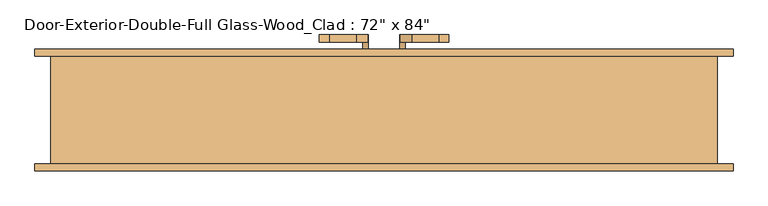
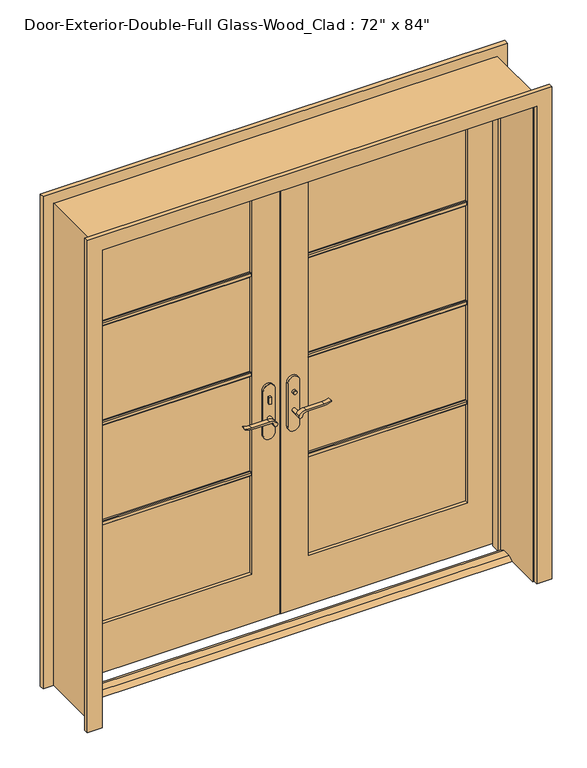
"""IFC4 building model written with IfcOpenShell, lengths in millimetres: door geometry."""

from ifc_helpers import new_model, si_unit, point, frame, frame_2d, origin, place, context, project, spatial, polyline, circle_curve, trimmed, segment, composite_curve, outline, extrude, faceted_brep, source, transform, mapped, element, save


def door_c1904fbe(model_context):
    return source(origin(), model_context, "Body", "SolidModel", [
        extrude(outline(polyline([(19.05, 12.7), (53.975, 12.7), (79.375, 0.0), (-6.35, 0.0), (19.05, 12.7)])), frame((-914.4, 0.0, 0.0), z_axis=(1.0, 0.0, 0.0), x_axis=(0.0, 1.0, 0.0)), (0.0, 0.0, 1.0), 1828.8),
        extrude(outline(polyline([(-47.4019111, 94.3), (-57.4019111, 94.3), (-57.4019111, 104.3), (-47.4019111, 104.3), (-47.4019111, 94.3)])), frame((0.0, 0.0, 981.9), z_axis=(0.0, 0.0, 1.0), x_axis=(1.0, 0.0, 0.0)), (0.0, 0.0, 1.0), 30.0),
        extrude(outline(composite_curve([segment(trimmed(circle_curve(frame_2d((996.9, -52.4019111)), 8.0), [point((996.9, -60.4019111))], [point((996.9, -44.4019111))], False, "CARTESIAN"), True, "CONTINUOUS"), segment(trimmed(circle_curve(frame_2d((996.9, -52.4019111)), 8.0), [point((996.9, -44.4019111))], [point((996.9, -60.4019111))], False, "CARTESIAN"), True, "CONTINUOUS")], self_intersect=False)), frame((0.0, 159.225, 0.0), z_axis=(0.0, 1.0, 0.0), x_axis=(0.0, 0.0, 1.0)), (0.0, 0.0, 1.0), 10.0),
        extrude(outline(composite_curve([segment(trimmed(circle_curve(frame_2d((897.1555521, -76.0694241)), 37.2832219), [point((919.0523287, -45.8937749))], [point((934.4, -77.7693445))], False, "CARTESIAN"), True, "CONTINUOUS"), segment(polyline([(934.4, -77.7693445), (934.4, -154.045502)]), True, "CONTINUOUS"), segment(trimmed(circle_curve(frame_2d((1017.6850638, -153.9791202)), 83.2850902), [point((934.4, -154.045502))], [point((939.4, -182.4019111))], True, "CARTESIAN"), True, "CONTINUOUS"), segment(polyline([(939.4, -182.4019111), (936.6135558, -182.4019111)]), True, "CONTINUOUS"), segment(trimmed(circle_curve(frame_2d((986.6709207, -150.4622499)), 59.3791355), [point((936.6135558, -182.4019111))], [point((927.4, -154.045502))], False, "CARTESIAN"), True, "CONTINUOUS"), segment(polyline([(927.4, -154.045502), (927.4, -77.7881013)]), True, "CONTINUOUS"), segment(trimmed(circle_curve(frame_2d((909.2738613, -77.7881013)), 18.1261387), [point((927.4, -77.7881013))], [point((914.4, -60.4019111))], True, "CARTESIAN"), True, "CONTINUOUS"), segment(trimmed(circle_curve(frame_2d((914.4, -52.4019111)), 8.0), [point((914.4, -60.4019111))], [point((919.0523287, -45.8937749))], False, "CARTESIAN"), True, "CONTINUOUS")], self_intersect=False)), frame((0.0, 54.3, 0.0), z_axis=(0.0, 1.0, 0.0), x_axis=(0.0, 0.0, 1.0)), (0.0, 0.0, 1.0), 20.0),
        extrude(outline(composite_curve([segment(trimmed(circle_curve(frame_2d((914.4, -52.4019111)), 8.0), [point((914.3999903, -60.4019111))], [point((919.0523287, -45.8937749))], False, "CARTESIAN"), True, "CONTINUOUS"), segment(trimmed(circle_curve(frame_2d((897.1555521, -76.0694241)), 37.2832219), [point((919.0523287, -45.8937749))], [point((934.4, -77.7693445))], False, "CARTESIAN"), True, "CONTINUOUS"), segment(polyline([(934.4, -77.7693445), (934.4, -154.045502)]), True, "CONTINUOUS"), segment(trimmed(circle_curve(frame_2d((1017.6850638, -153.9791202)), 83.2850902), [point((934.4, -154.045502))], [point((939.4, -182.4019111))], True, "CARTESIAN"), True, "CONTINUOUS"), segment(polyline([(939.4, -182.4019111), (936.6135558, -182.4019111)]), True, "CONTINUOUS"), segment(trimmed(circle_curve(frame_2d((986.6709207, -150.4622499)), 59.3791355), [point((936.6135558, -182.4019111))], [point((927.4, -154.045502))], False, "CARTESIAN"), True, "CONTINUOUS"), segment(polyline([(927.4, -154.045502), (927.4, -77.788099)]), True, "CONTINUOUS"), segment(trimmed(circle_curve(frame_2d((909.2738682, -77.788099)), 18.1261318), [point((927.4, -77.788099))], [point((914.3999903, -60.4019111))], True, "CARTESIAN"), True, "CONTINUOUS")], self_intersect=False)), frame((0.0, 189.225, 0.0), z_axis=(0.0, 1.0, 0.0), x_axis=(0.0, 0.0, 1.0)), (0.0, 0.0, 1.0), 20.0),
        extrude(outline(composite_curve([segment(trimmed(circle_curve(frame_2d((914.4, -52.4019111)), 8.0), [point((914.4, -60.4019111))], [point((914.4, -44.4019111))], False, "CARTESIAN"), True, "CONTINUOUS"), segment(trimmed(circle_curve(frame_2d((914.4, -52.4019111)), 8.0), [point((914.4, -44.4019111))], [point((914.4, -60.4019111))], False, "CARTESIAN"), True, "CONTINUOUS")], self_intersect=False)), frame((0.0, 74.3, 0.0), z_axis=(0.0, 1.0, 0.0), x_axis=(0.0, 0.0, 1.0)), (0.0, 0.0, 1.0), 30.0),
        extrude(outline(composite_curve([segment(trimmed(circle_curve(frame_2d((914.4, -52.4019111)), 8.0), [point((914.4, -60.4019111))], [point((914.4, -44.4019111))], False, "CARTESIAN"), True, "CONTINUOUS"), segment(trimmed(circle_curve(frame_2d((914.4, -52.4019111)), 8.0), [point((914.4, -44.4019111))], [point((914.4, -60.4019111))], False, "CARTESIAN"), True, "CONTINUOUS")], self_intersect=False)), frame((0.0, 159.225, 0.0), z_axis=(0.0, 1.0, 0.0), x_axis=(0.0, 0.0, 1.0)), (0.0, 0.0, 1.0), 30.0),
        extrude(outline(composite_curve([segment(polyline([(844.4, -27.4019111), (1039.4, -27.4019111)]), True, "CONTINUOUS"), segment(trimmed(circle_curve(frame_2d((1039.4, -52.4019111)), 25.0), [point((1039.4, -27.4019111))], [point((1039.4, -77.4019111))], False, "CARTESIAN"), True, "CONTINUOUS"), segment(polyline([(1039.4, -77.4019111), (844.4, -77.4019111)]), True, "CONTINUOUS"), segment(trimmed(circle_curve(frame_2d((844.4, -52.4019111)), 25.0), [point((844.4, -77.4019111))], [point((844.4, -27.4019111))], False, "CARTESIAN"), True, "CONTINUOUS")], self_intersect=False)), frame((0.0, 104.3, 0.0), z_axis=(0.0, 1.0, 0.0), x_axis=(0.0, 0.0, 1.0)), (0.0, 0.0, 1.0), 10.0),
        extrude(outline(composite_curve([segment(polyline([(844.4, -27.4019111), (1039.4, -27.4019111)]), True, "CONTINUOUS"), segment(trimmed(circle_curve(frame_2d((1039.4, -52.4019111)), 25.0), [point((1039.4, -27.4019111))], [point((1039.4, -77.4019111))], False, "CARTESIAN"), True, "CONTINUOUS"), segment(polyline([(1039.4, -77.4019111), (844.4, -77.4019111)]), True, "CONTINUOUS"), segment(trimmed(circle_curve(frame_2d((844.4, -52.4019111)), 25.0), [point((844.4, -77.4019111))], [point((844.4, -27.4019111))], False, "CARTESIAN"), True, "CONTINUOUS")], self_intersect=False)), frame((0.0, 149.225, 0.0), z_axis=(0.0, 1.0, 0.0), x_axis=(0.0, 0.0, 1.0)), (0.0, 0.0, 1.0), 10.0),
        extrude(outline(polyline([(47.3875, 169.225), (57.3875, 169.225), (57.3875, 159.225), (47.3875, 159.225), (47.3875, 169.225)])), frame((0.0, 0.0, 981.9), z_axis=(0.0, 0.0, 1.0), x_axis=(1.0, 0.0, 0.0)), (0.0, 0.0, 1.0), 30.0),
        extrude(outline(composite_curve([segment(trimmed(circle_curve(frame_2d((996.9, 52.3875)), 8.0), [point((996.9, 60.3875))], [point((996.9, 44.3875))], False, "CARTESIAN"), True, "CONTINUOUS"), segment(trimmed(circle_curve(frame_2d((996.9, 52.3875)), 8.0), [point((996.9, 44.3875))], [point((996.9, 60.3875))], False, "CARTESIAN"), True, "CONTINUOUS")], self_intersect=False)), frame((0.0, 94.3, 0.0), z_axis=(0.0, 1.0, 0.0), x_axis=(0.0, 0.0, 1.0)), (0.0, 0.0, 1.0), 10.0),
        extrude(outline(composite_curve([segment(trimmed(circle_curve(frame_2d((914.4, 52.3875)), 8.0), [point((919.0523287, 45.8793637))], [point((914.4, 60.3875))], False, "CARTESIAN"), True, "CONTINUOUS"), segment(trimmed(circle_curve(frame_2d((909.2738613, 77.7736901)), 18.1261387), [point((914.4, 60.3875))], [point((927.4, 77.7736901))], True, "CARTESIAN"), True, "CONTINUOUS"), segment(polyline([(927.4, 77.7736901), (927.4, 154.0310909)]), True, "CONTINUOUS"), segment(trimmed(circle_curve(frame_2d((986.6709207, 150.4478388)), 59.3791355), [point((927.4, 154.0310909))], [point((936.6135558, 182.3875))], False, "CARTESIAN"), True, "CONTINUOUS"), segment(polyline([(936.6135558, 182.3875), (939.4, 182.3875)]), True, "CONTINUOUS"), segment(trimmed(circle_curve(frame_2d((1017.6850638, 153.9647091)), 83.2850902), [point((939.4, 182.3875))], [point((934.4, 154.0310909))], True, "CARTESIAN"), True, "CONTINUOUS"), segment(polyline([(934.4, 154.0310909), (934.4, 77.7549333)]), True, "CONTINUOUS"), segment(trimmed(circle_curve(frame_2d((897.1555521, 76.0550129)), 37.2832219), [point((934.4, 77.7549333))], [point((919.0523287, 45.8793637))], False, "CARTESIAN"), True, "CONTINUOUS")], self_intersect=False)), frame((0.0, 189.225, 0.0), z_axis=(0.0, 1.0, 0.0), x_axis=(0.0, 0.0, 1.0)), (0.0, 0.0, 1.0), 20.0),
        extrude(outline(composite_curve([segment(trimmed(circle_curve(frame_2d((909.2738682, 77.7736878)), 18.1261318), [point((914.3999903, 60.3875))], [point((927.4, 77.7736878))], True, "CARTESIAN"), True, "CONTINUOUS"), segment(polyline([(927.4, 77.7736878), (927.4, 154.0310909)]), True, "CONTINUOUS"), segment(trimmed(circle_curve(frame_2d((986.6709207, 150.4478388)), 59.3791355), [point((927.4, 154.0310909))], [point((936.6135558, 182.3875))], False, "CARTESIAN"), True, "CONTINUOUS"), segment(polyline([(936.6135558, 182.3875), (939.4, 182.3875)]), True, "CONTINUOUS"), segment(trimmed(circle_curve(frame_2d((1017.6850638, 153.9647091)), 83.2850902), [point((939.4, 182.3875))], [point((934.4, 154.0310909))], True, "CARTESIAN"), True, "CONTINUOUS"), segment(polyline([(934.4, 154.0310909), (934.4, 77.7549333)]), True, "CONTINUOUS"), segment(trimmed(circle_curve(frame_2d((897.1555521, 76.0550129)), 37.2832219), [point((934.4, 77.7549333))], [point((919.0523287, 45.8793637))], False, "CARTESIAN"), True, "CONTINUOUS"), segment(trimmed(circle_curve(frame_2d((914.4, 52.3875)), 8.0), [point((919.0523287, 45.8793637))], [point((914.3999903, 60.3875))], False, "CARTESIAN"), True, "CONTINUOUS")], self_intersect=False)), frame((0.0, 54.3, 0.0), z_axis=(0.0, 1.0, 0.0), x_axis=(0.0, 0.0, 1.0)), (0.0, 0.0, 1.0), 20.0),
        extrude(outline(composite_curve([segment(trimmed(circle_curve(frame_2d((914.4, 52.3875)), 8.0), [point((914.4, 60.3875))], [point((914.4, 44.3875))], False, "CARTESIAN"), True, "CONTINUOUS"), segment(trimmed(circle_curve(frame_2d((914.4, 52.3875)), 8.0), [point((914.4, 44.3875))], [point((914.4, 60.3875))], False, "CARTESIAN"), True, "CONTINUOUS")], self_intersect=False)), frame((0.0, 159.225, 0.0), z_axis=(0.0, 1.0, 0.0), x_axis=(0.0, 0.0, 1.0)), (0.0, 0.0, 1.0), 30.0),
        extrude(outline(composite_curve([segment(trimmed(circle_curve(frame_2d((914.4, 52.3875)), 8.0), [point((914.4, 60.3875))], [point((914.4, 44.3875))], False, "CARTESIAN"), True, "CONTINUOUS"), segment(trimmed(circle_curve(frame_2d((914.4, 52.3875)), 8.0), [point((914.4, 44.3875))], [point((914.4, 60.3875))], False, "CARTESIAN"), True, "CONTINUOUS")], self_intersect=False)), frame((0.0, 74.3, 0.0), z_axis=(0.0, 1.0, 0.0), x_axis=(0.0, 0.0, 1.0)), (0.0, 0.0, 1.0), 30.0),
        extrude(outline(composite_curve([segment(trimmed(circle_curve(frame_2d((844.4, 52.3875)), 25.0), [point((844.4, 27.3875))], [point((844.4, 77.3875))], False, "CARTESIAN"), True, "CONTINUOUS"), segment(polyline([(844.4, 77.3875), (1039.4, 77.3875)]), True, "CONTINUOUS"), segment(trimmed(circle_curve(frame_2d((1039.4, 52.3875)), 25.0), [point((1039.4, 77.3875))], [point((1039.4, 27.3875))], False, "CARTESIAN"), True, "CONTINUOUS"), segment(polyline([(1039.4, 27.3875), (844.4, 27.3875)]), True, "CONTINUOUS")], self_intersect=False)), frame((0.0, 149.225, 0.0), z_axis=(0.0, 1.0, 0.0), x_axis=(0.0, 0.0, 1.0)), (0.0, 0.0, 1.0), 10.0),
        extrude(outline(composite_curve([segment(trimmed(circle_curve(frame_2d((844.4, 52.3875)), 25.0), [point((844.4, 27.3875))], [point((844.4, 77.3875))], False, "CARTESIAN"), True, "CONTINUOUS"), segment(polyline([(844.4, 77.3875), (1039.4, 77.3875)]), True, "CONTINUOUS"), segment(trimmed(circle_curve(frame_2d((1039.4, 52.3875)), 25.0), [point((1039.4, 77.3875))], [point((1039.4, 27.3875))], False, "CARTESIAN"), True, "CONTINUOUS"), segment(polyline([(1039.4, 27.3875), (844.4, 27.3875)]), True, "CONTINUOUS")], self_intersect=False)), frame((0.0, 104.3, 0.0), z_axis=(0.0, 1.0, 0.0), x_axis=(0.0, 0.0, 1.0)), (0.0, 0.0, 1.0), 10.0),
        extrude(outline(polyline([(128.27, 1578.371875), (128.27, 1559.321875), (121.92, 1559.321875), (118.745, 1562.496875), (118.745, 1575.196875), (121.92, 1578.371875), (128.27, 1578.371875)])), frame((120.65, 0.0, 0.0), z_axis=(1.0, 0.0, 0.0), x_axis=(0.0, 1.0, 0.0)), (0.0, 0.0, 1.0), 673.1),
        extrude(outline(polyline([(128.27, 1132.68125), (128.27, 1113.63125), (121.92, 1113.63125), (118.745, 1116.80625), (118.745, 1129.50625), (121.92, 1132.68125), (128.27, 1132.68125)])), frame((120.65, 0.0, 0.0), z_axis=(1.0, 0.0, 0.0), x_axis=(0.0, 1.0, 0.0)), (0.0, 0.0, 1.0), 673.1),
        extrude(outline(polyline([(128.27, 686.990625), (128.27, 667.940625), (121.92, 667.940625), (118.745, 671.115625), (118.745, 683.815625), (121.92, 686.990625), (128.27, 686.990625)])), frame((120.65, 0.0, 0.0), z_axis=(1.0, 0.0, 0.0), x_axis=(0.0, 1.0, 0.0)), (0.0, 0.0, 1.0), 673.1),
        extrude(outline(polyline([(135.255, 1578.371875), (141.605, 1578.371875), (144.78, 1575.196875), (144.78, 1562.496875), (141.605, 1559.321875), (135.255, 1559.321875), (135.255, 1578.371875)])), frame((-793.75, 0.0, 0.0), z_axis=(1.0, 0.0, 0.0), x_axis=(0.0, 1.0, 0.0)), (0.0, 0.0, 1.0), 673.1),
        extrude(outline(polyline([(135.255, 1132.68125), (141.605, 1132.68125), (144.78, 1129.50625), (144.78, 1116.80625), (141.605, 1113.63125), (135.255, 1113.63125), (135.255, 1132.68125)])), frame((-793.75, 0.0, 0.0), z_axis=(1.0, 0.0, 0.0), x_axis=(0.0, 1.0, 0.0)), (0.0, 0.0, 1.0), 673.1),
        extrude(outline(polyline([(135.255, 686.990625), (141.605, 686.990625), (144.78, 683.815625), (144.78, 671.115625), (141.605, 667.940625), (135.255, 667.940625), (135.255, 686.990625)])), frame((-793.75, 0.0, 0.0), z_axis=(1.0, 0.0, 0.0), x_axis=(0.0, 1.0, 0.0)), (0.0, 0.0, 1.0), 673.1),
        extrude(outline(polyline([(135.255, 1578.371875), (141.605, 1578.371875), (144.78, 1575.196875), (144.78, 1562.496875), (141.605, 1559.321875), (135.255, 1559.321875), (135.255, 1578.371875)])), frame((120.65, 0.0, 0.0), z_axis=(1.0, 0.0, 0.0), x_axis=(0.0, 1.0, 0.0)), (0.0, 0.0, 1.0), 673.1),
        extrude(outline(polyline([(135.255, 1132.68125), (141.605, 1132.68125), (144.78, 1129.50625), (144.78, 1116.80625), (141.605, 1113.63125), (135.255, 1113.63125), (135.255, 1132.68125)])), frame((120.65, 0.0, 0.0), z_axis=(1.0, 0.0, 0.0), x_axis=(0.0, 1.0, 0.0)), (0.0, 0.0, 1.0), 673.1),
        extrude(outline(polyline([(135.255, 686.990625), (141.605, 686.990625), (144.78, 683.815625), (144.78, 671.115625), (141.605, 667.940625), (135.255, 667.940625), (135.255, 686.990625)])), frame((120.65, 0.0, 0.0), z_axis=(1.0, 0.0, 0.0), x_axis=(0.0, 1.0, 0.0)), (0.0, 0.0, 1.0), 673.1),
        extrude(outline(polyline([(128.27, 1578.371875), (128.27, 1559.321875), (121.92, 1559.321875), (118.745, 1562.496875), (118.745, 1575.196875), (121.92, 1578.371875), (128.27, 1578.371875)])), frame((-793.75, 0.0, 0.0), z_axis=(1.0, 0.0, 0.0), x_axis=(0.0, 1.0, 0.0)), (0.0, 0.0, 1.0), 673.1),
        extrude(outline(polyline([(128.27, 1132.68125), (128.27, 1113.63125), (121.92, 1113.63125), (118.745, 1116.80625), (118.745, 1129.50625), (121.92, 1132.68125), (128.27, 1132.68125)])), frame((-793.75, 0.0, 0.0), z_axis=(1.0, 0.0, 0.0), x_axis=(0.0, 1.0, 0.0)), (0.0, 0.0, 1.0), 673.1),
        extrude(outline(polyline([(128.27, 686.990625), (128.27, 667.940625), (121.92, 667.940625), (118.745, 671.115625), (118.745, 683.815625), (121.92, 686.990625), (128.27, 686.990625)])), frame((-793.75, 0.0, 0.0), z_axis=(1.0, 0.0, 0.0), x_axis=(0.0, 1.0, 0.0)), (0.0, 0.0, 1.0), 673.1),
        extrude(outline(polyline([(0.0, 920.75), (0.0, 984.25), (2203.45, 984.25), (2203.45, -984.25), (0.0, -984.25), (0.0, -920.75), (2139.95, -920.75), (2139.95, 920.75), (0.0, 920.75)])), frame((0.0, -174.625, 0.0), z_axis=(0.0, 1.0, 0.0), x_axis=(0.0, 0.0, 1.0)), (0.0, 0.0, 1.0), 19.05),
        extrude(outline(polyline([(0.0, 920.75), (0.0, 984.25), (2203.45, 984.25), (2203.45, -984.25), (0.0, -984.25), (0.0, -920.75), (2139.95, -920.75), (2139.95, 920.75), (0.0, 920.75)])), frame((0.0, 149.225, 0.0), z_axis=(0.0, 1.0, 0.0), x_axis=(0.0, 0.0, 1.0)), (0.0, 0.0, 1.0), 19.05),
        faceted_brep([(939.8, 149.225, 0.0), (939.8, -155.575, 0.0), (914.4, -155.575, 0.0), (914.4, 79.375, 0.0), (901.7, 79.375, 0.0), (901.7, 114.3, 0.0), (914.4, 114.3, 0.0), (914.4, 149.225, 0.0), (939.8, 149.225, 2159.0), (939.8, -155.575, 2159.0), (-939.8, -155.575, 2159.0), (-939.8, -155.575, 0.0), (-914.4, -155.575, 0.0), (-914.4, -155.575, 2133.6), (914.4, -155.575, 2133.6), (914.4, 79.375, 2133.6), (-914.4, 79.375, 2133.6), (-914.4, 79.375, 0.0), (-901.7, 79.375, 0.0), (-901.7, 79.375, 2120.9), (901.7, 79.375, 2120.9), (901.7, 114.3, 2120.9), (1.5875, 114.3, 2120.9), (-1.6019111, 114.3, 2120.9), (-901.7, 114.3, 2120.9), (-901.7, 114.3, 0.0), (-914.4, 114.3, 0.0), (-914.4, 114.3, 2133.6), (-1.6019111, 114.3, 2133.6), (1.5875, 114.3, 2133.6), (914.4, 114.3, 2133.6), (914.4, 149.225, 2133.6), (1.5875, 149.225, 2133.6), (-1.6019111, 149.225, 2133.6), (-914.4, 149.225, 2133.6), (-914.4, 149.225, 0.0), (-939.8, 149.225, 0.0), (-939.8, 149.225, 2159.0)], [[[0, 1, 2, 3, 4, 5, 6, 7]], [[1, 0, 8, 9]], [[2, 1, 9, 10, 11, 12, 13, 14]], [[3, 2, 14, 15]], [[4, 3, 15, 16, 17, 18, 19, 20]], [[5, 4, 20, 21]], [[6, 5, 21, 22, 23, 24, 25, 26, 27, 28, 29, 30]], [[7, 6, 30, 31]], [[0, 7, 31, 32, 33, 34, 35, 36, 37, 8]], [[9, 8, 37, 10]], [[14, 13, 16, 15]], [[20, 19, 24, 23, 22, 21]], [[31, 30, 29, 28, 27, 34, 33, 32]], [[12, 11, 36, 35, 26, 25, 18, 17]], [[11, 10, 37, 36]], [[13, 12, 17, 16]], [[19, 18, 25, 24]], [[27, 26, 35, 34]]]),
        extrude(outline(polyline([(12.7, 914.4), (2133.6, 914.4), (2133.6, 1.5875), (12.7, 1.5875), (12.7, 914.4)]), holes=[polyline([(2014.5375, 120.65), (2014.5375, 793.75), (231.775, 793.75), (231.775, 120.65), (2014.5375, 120.65)])]), frame((0.0, 114.3, 0.0), z_axis=(0.0, 1.0, 0.0), x_axis=(0.0, 0.0, 1.0)), (0.0, 0.0, 1.0), 34.925),
        extrude(outline(polyline([(2133.6, -914.4), (12.7, -914.4), (12.7, -1.6019111), (2133.6, -1.6019111), (2133.6, -914.4)]), holes=[polyline([(231.775, -793.75), (2014.5375, -793.75), (2014.5375, -120.65), (231.775, -120.65), (231.775, -793.75)])]), frame((0.0, 114.3, 0.0), z_axis=(0.0, 1.0, 0.0), x_axis=(0.0, 0.0, 1.0)), (0.0, 0.0, 1.0), 34.925),
        extrude(outline(polyline([(793.75, 128.27), (120.65, 128.27), (120.65, 135.255), (793.75, 135.255), (793.75, 128.27)])), frame((0.0, 0.0, 231.775), z_axis=(0.0, 0.0, 1.0), x_axis=(1.0, 0.0, 0.0)), (0.0, 0.0, 1.0), 1782.7625),
        extrude(outline(polyline([(-120.65, 128.27), (-793.75, 128.27), (-793.75, 135.255), (-120.65, 135.255), (-120.65, 128.27)])), frame((0.0, 0.0, 231.775), z_axis=(0.0, 0.0, 1.0), x_axis=(1.0, 0.0, 0.0)), (0.0, 0.0, 1.0), 1782.7625),
    ])


if __name__ == "__main__":
    model = new_model("IFC4")
    model_context = context("Model", 3, world=origin())
    ifc_project = project(units=[si_unit("LENGTHUNIT", "METRE", prefix="MILLI")], contexts=[model_context])
    site = spatial("IfcSite", under=ifc_project)
    building = spatial("IfcBuilding", under=site)
    placement = place(None, origin())
    door_shape = door_c1904fbe(model_context)
    element("IfcDoor", 1, ObjectType="Door-Exterior-Double-Full Glass-Wood_Clad : 72\" x 84\"", at=placement, inside=building, context=model_context, shape_type="MappedRepresentation", body=[
        mapped(door_shape, transform((0.0, 0.0, 0.0), x_axis=(1.0, 0.0, 0.0), y_axis=(0.0, 1.0, 0.0), z_axis=(0.0, 0.0, 1.0))),
    ])
    save(model, "model.ifc")

# Revit data of these elements
# Type "Door-Exterior-Double-Full Glass-Wood_Clad : 72\" x 84\""
#   Type Mark = "13"
#   Assembly Code = "B2030100"
#   Analytic Construction = "French door, wood frame with double glass"
#   Top Rail = 0' - 4 11/16"
#   Threshold Offset [instance default] = 0' - 0 1/2"
#   Thickness = 0' - 1 3/8"
#   Thermal Resistance (R) = 1.9158 (h·ft²·°F)/BTU
#   Swing Angle [instance default] = 90.00°
#   Stiles = 0' - 4 3/4"
#   Rough Width = 6' - 2"
#   Rough Height = 7' - 1"
#   Panel Width = 3' - 0"
#   Door Offset [instance default] = 0' - 0"
#   Height = 7' - 0"
#   Width = 6' - 0"
#   Heat Transfer Coefficient (U) = 0.5220 BTU/(h·ft²·°F)
#   Bottom Rail = 0' - 9 1/8"
#   Exterior Trim [instance default] = yes
#   Threshold [instance default] = yes
#   Show Grill [instance default] = yes
#   Function = 1
#   Trim Material = Cherry
#   Threshold Material = Cherry
#   Panel Material = Cherry
#   Glazing = Glass
#   Frame Material = Cherry
#   Door Handle Material = Aluminum
#   Visual Light Transmittance = 0
#   Solar Heat Gain Coefficient = 0
#   Wall Closure = (empty or 0)
#   Construction Type = (empty or 0)
# Element 1 (IfcDoor, "Door-Exterior-Double-Full Glass-Wood_Clad : 72\" x 84\"")
#   Materials on its faces: "Cherry", "Aluminum", "Glass"
# Materials
#   "Cherry": class "Wood", colour RGB 226 177 128, transparency 0, Description = "Prunus Serotina", Cost = 0
#   "Glass": class "Glass", colour RGB 0 128 192, transparency 0.75, Description = "Soda Lime Glass", Cost = 0
#   "Aluminum": class "Metal", colour RGB 247 247 247, transparency 0, Description = "Aluminum 6061", Cost = 0
